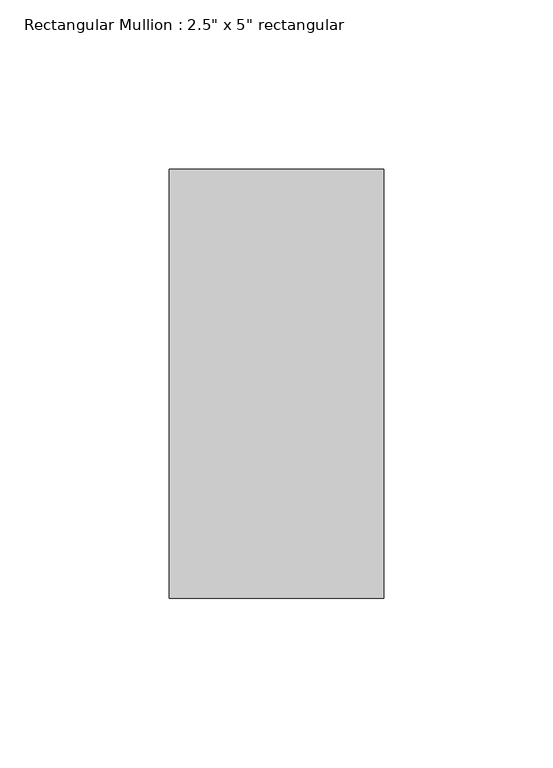
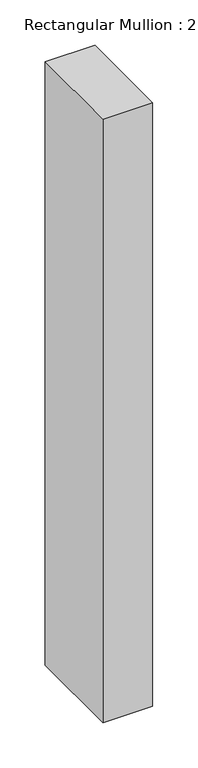
"""IFC4 building model written with IfcOpenShell, lengths in millimetres: member geometry."""

from ifc_helpers import new_model, si_unit, frame, origin, place, context, project, spatial, polyline, outline, extrude, source, transform, mapped, element, save


def member_1f059faf(model_context):
    return source(origin(), model_context, "Body", "SweptSolid", [
        extrude(outline(polyline([(0.0, 63.5), (0.0, -63.5), (-63.5, -63.5), (-63.5, 63.5), (0.0, 63.5)])), frame((0.0, 0.0, -811.4673296), z_axis=(0.0, 0.0, 1.0), x_axis=(1.0, 0.0, 0.0)), (0.0, 0.0, 1.0), 811.4673296),
    ])


if __name__ == "__main__":
    model = new_model("IFC4")
    model_context = context("Model", 3, world=origin())
    ifc_project = project(units=[si_unit("LENGTHUNIT", "METRE", prefix="MILLI")], contexts=[model_context])
    site = spatial("IfcSite", under=ifc_project)
    building = spatial("IfcBuilding", under=site)
    placement = place(None, origin())
    member_shape = member_1f059faf(model_context)
    element("IfcMember", 1, ObjectType="Rectangular Mullion : 2.5\" x 5\" rectangular", at=placement, inside=building, context=model_context, shape_type="MappedRepresentation", body=[
        mapped(member_shape, transform((0.0, 0.0, 0.0), x_axis=(1.0, 0.0, 0.0), y_axis=(0.0, 1.0, 0.0), z_axis=(0.0, 0.0, 1.0))),
    ])
    save(model, "model.ifc")

# Revit data of these elements
# Type "Rectangular Mullion : 2.5\" x 5\" rectangular"
#   built-in parameter 1007304 = 0.416667 (stored number, unit not read)
#   built-in parameter 1007301 = 0.104167 (stored number, unit not read)
#   built-in parameter 1007300 = 0.104167 (stored number, unit not read)
# Element 1 (IfcMember, "Rectangular Mullion : 2.5\" x 5\" rectangular")
#   Materials on its faces: "Aluminum"
# Materials
#   "Aluminum": class "Metal", colour RGB 247 247 247, transparency 0, Description = "Aluminum 6061", Cost = 0
